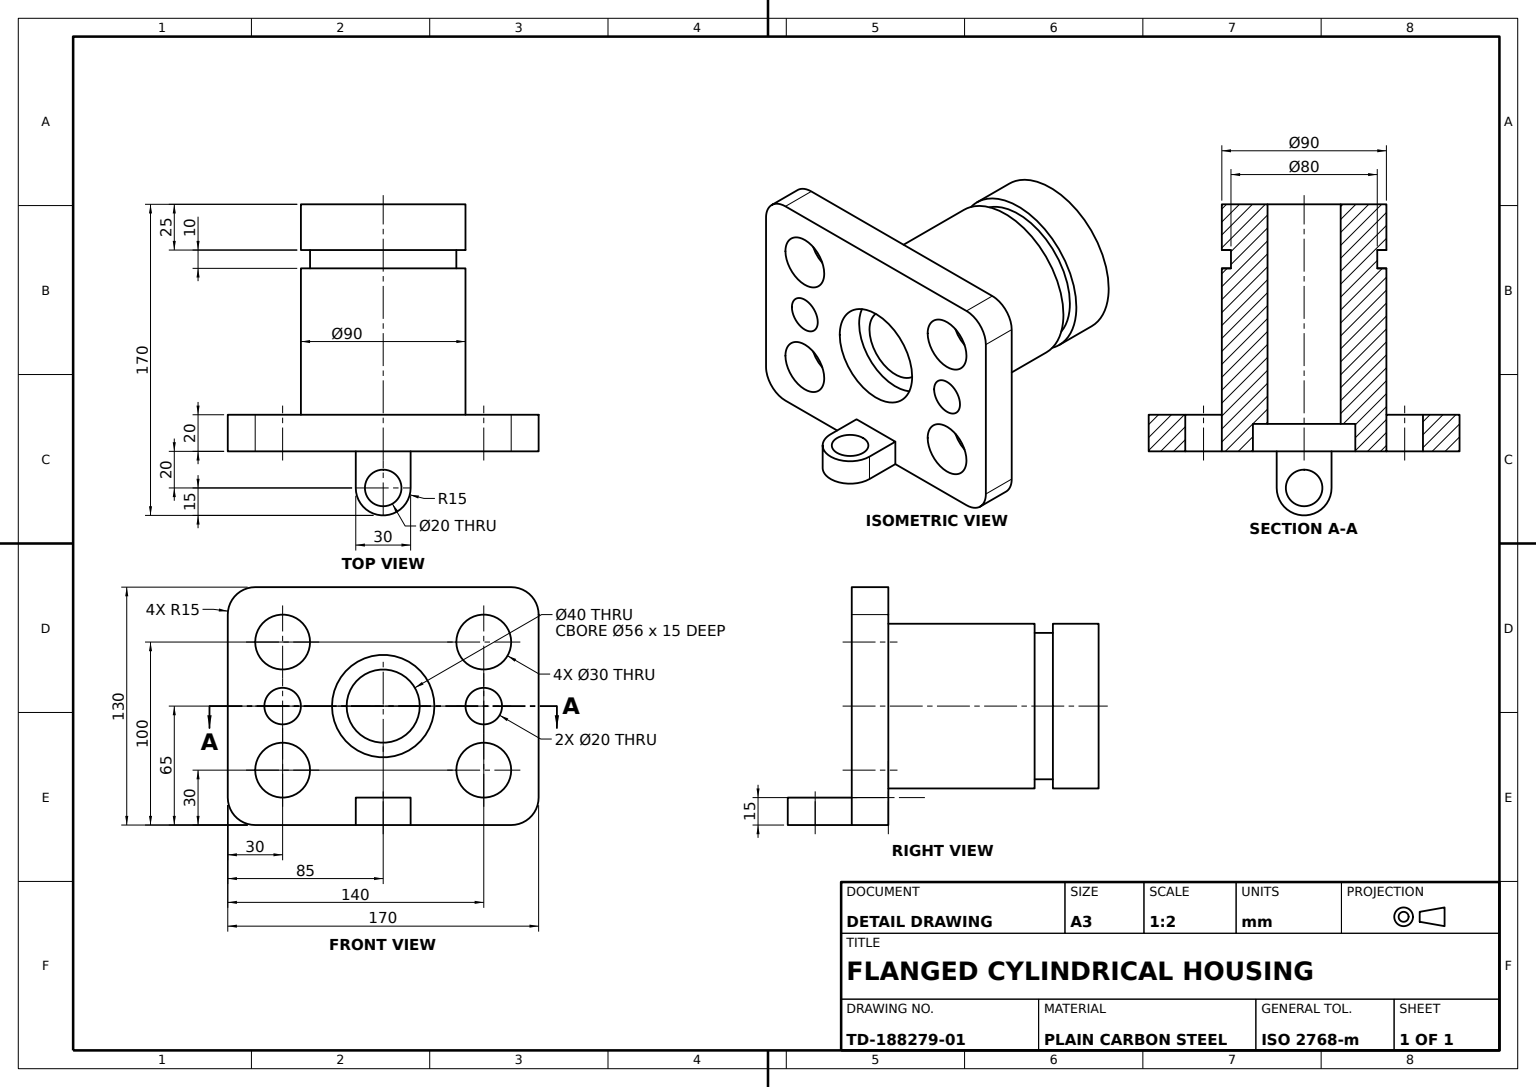
SolidWorks part; units mm, degrees
material "Plain Carbon Steel"
ref_plane "Front Plane" through (0, 0, 0) normal (0, 0, 1) x (1, 0, 0)
ref_plane "Top Plane" through (0, 0, 0) normal (0, 1, 0) x (1, 0, 0)
ref_plane "Right Plane" through (0, 0, 0) normal (1, 0, 0) x (0, 0, -1)
sketch "Column Base Sketch" plane through (0, 0, 0) normal (0, 0, 1) x (1, 0, 0)
  circle A0 centre (0, 0) radius 45
  dimension "D1" = 90
extrude "Column Base Ø90" add sketch "Column Base Sketch" along normal blind 25
sketch "Groove Neck Sketch" plane through (0, 0, 25) normal (0, 0, 1) x (1, 0, 0)
  circle A0 centre (0, 0) radius 40
  dimension "D1" = 80
extrude "Groove Neck Ø80" add sketch "Groove Neck Sketch" along normal blind 10
sketch "Column Body Sketch" plane through (0, 0, 35) normal (0, 0, 1) x (1, 0, 0)
  circle A0 centre (0, 0) radius 45
  dimension "D1" = 90
extrude "Column Body Ø90" add sketch "Column Body Sketch" along normal blind 80
sketch "Top Plate Sketch" plane through (0, 0, 115) normal (0, 0, 1) x (1, 0, 0)
  line L0 (0, 0) -> (0, 65)
  line L1 (0, 65) -> (70, 65)
  line L2 (85, 50) -> (85, -50)
  line L3 (70, -65) -> (-70, -65)
  line L4 (-85, -50) -> (-85, 50)
  line L5 (-70, 65) -> (0, 65)
  arc A0 (-70, -65) -> (-85, -50) centre (-70, -50) cw
  arc A1 (70, -65) -> (85, -50) centre (70, -50) ccw
  arc A2 (85, 50) -> (70, 65) centre (70, 50) ccw
  arc A3 (-70, 65) -> (-85, 50) centre (-70, 50) ccw
  point P9 (-85, -65)
  point P12 (85, -65)
  point P15 (85, 65)
  point P18 (-85, 65)
  dimension "D6" = 15
  dimension "D1" = 65
  dimension "D2" = 85
  dimension "D3" = 130
  dimension "D4" = 170
  dimension "D5" = 130
extrude "Top Plate 170x130" add sketch "Top Plate Sketch" along normal blind 20
sketch "Bore Step Sketch" plane through (0, 0, 135) normal (0, 0, 1) x (1, 0, 0)
  circle A0 centre (0, 0) radius 28
  dimension "D1" = 28
extrude "Bore Step Ø28" cut sketch "Bore Step Sketch" against normal blind 15
sketch "Column Bore Sketch" plane through (0, 0, 120) normal (0, 0, 1) x (1, 0, 0)
  circle A0 centre (0, 0) radius 20
  dimension "D1" = 40
extrude "Column Bore Ø40" cut sketch "Column Bore Sketch" against normal blind 150
sketch "Plate Holes Sketch" plane through (0, 0, 135) normal (0, 0, 1) x (1, 0, 0)
  line L0 (-85, 0) -> (-55, 0)
  line L1 (-85, -50) -> (-85, 50) construction
  line L2 (85, 0) -> (55, 0)
  line L3 (85, 50) -> (85, -50) construction
  line L4 (-55, 65) -> (-55, 35)
  line L5 (-70, 65) -> (70, 65) construction
  line L6 (55, 65) -> (55, 35)
  line L7 (-55, -65) -> (-55, -35)
  line L8 (70, -65) -> (-70, -65) construction
  line L9 (55, -65) -> (55, -35)
  circle A0 centre (-55, 35) radius 15
  circle A1 centre (55, 35) radius 15
  circle A2 centre (-55, -35) radius 15
  circle A3 centre (55, -35) radius 15
  circle A4 centre (-55, 0) radius 10
  circle A5 centre (55, 0) radius 10
  dimension "D1" = 30
  dimension "D7" = 15
  dimension "D8" = 15
  dimension "D9" = 15
  dimension "D10" = 15
  dimension "D11" = 10
  dimension "D12" = 10
  dimension "D2" = 30
  dimension "D3" = 30
  dimension "D4" = 30
  dimension "D5" = 30
  dimension "D6" = 30
extrude "Plate Holes 6x" cut sketch "Plate Holes Sketch" against normal blind 150
sketch "Eye Lug Sketch" plane through (0, -65, 0) normal (0, -1, 0) x (1, 0, 0)
  line L0 (-15, 135) -> (15, 135)
  line L1 (70, 135) -> (-70, 135) construction
  line L2 (15, 155) -> (15, 135)
  line L3 (-15, 155) -> (-15, 135)
  arc A0 (15, 155) -> (-15, 155) centre (0, 155) ccw
  dimension "D2" = 15
  dimension "D3" = 55
  dimension "D1" = 20
extrude "Eye Lug" add sketch "Eye Lug Sketch" against normal blind 15
sketch "Lug Hole Sketch" plane through (0, -50, 0) normal (0, 1, 0) x (1, 0, 0)
  circle A0 centre (0, -155) radius 10
  dimension "D1" = 10
extrude "Lug Hole Ø10" cut sketch "Lug Hole Sketch" against normal blind 15
